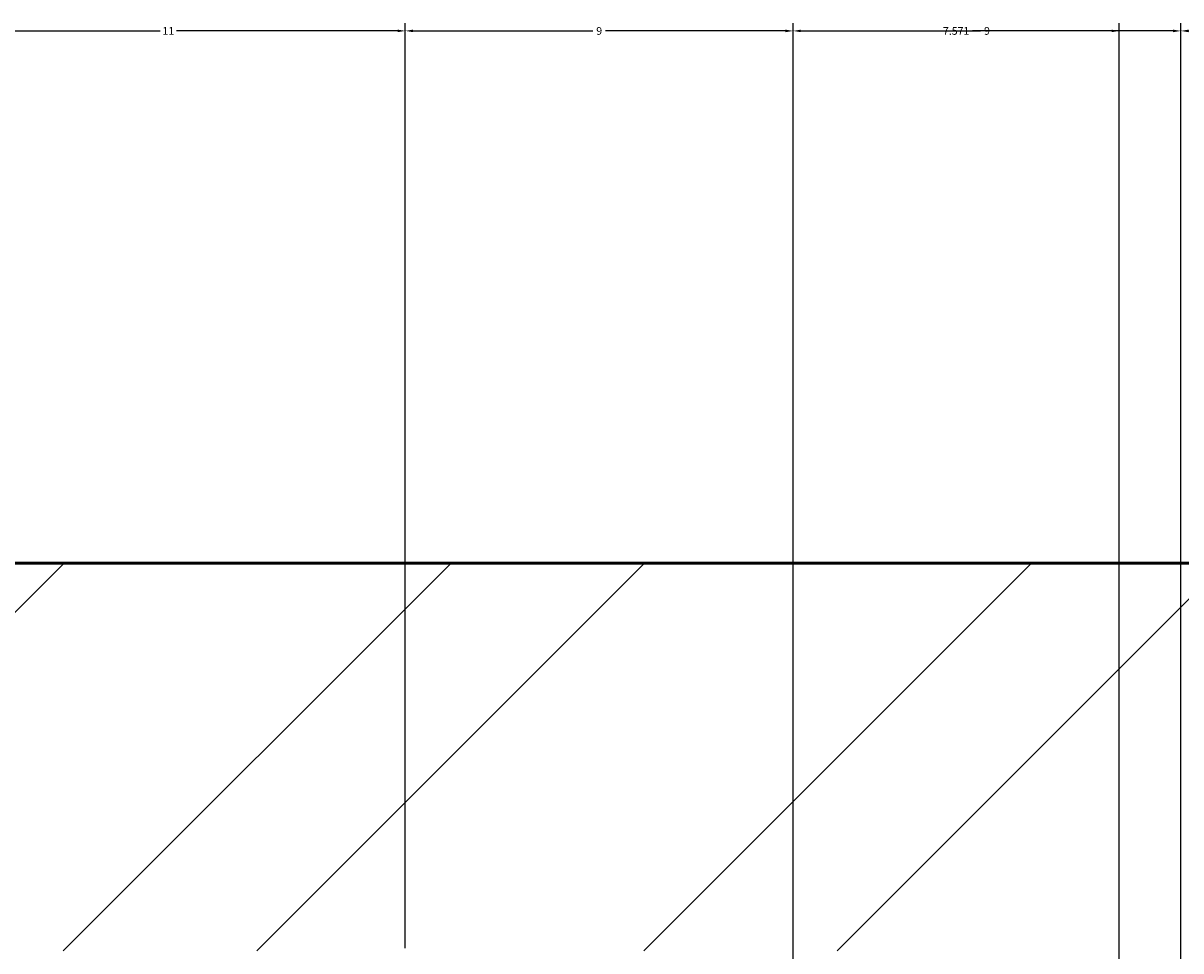
# Model space of a CAD drawing. Units: inches. Extents: x 2812 to 3051, y 1398 to 1659.
# Tile 63 of 65: x 2944 to 2970, y 1638 to 1659. Entities that reach past the tile are written whole.
import ezdxf

# ---------------------------------------------------------------- set-up
doc = ezdxf.new("R2010")
doc.units = ezdxf.units.IN
for name, color, linetype, lineweight in [('A-ANNO-DIMS', 2, 'Continuous', 18), ('S-CONC', 7, 'Continuous', 50), ('S-CONC-PATT', 8, 'Continuous', 18)]:
    doc.layers.add(name, color=color, linetype=linetype, lineweight=lineweight)
doc.styles.get("Standard").update_dxf_attribs({"font": 'arial.ttf'})
doc.dimstyles.get("Standard").update_dxf_attribs({"dimtxt": 0.18, "dimasz": 0.18, "dimexe": 0.18, "dimexo": 0.0625, "dimgap": 0.09, "dimtad": 0, "dimtih": 1, "dimtoh": 1, "dimdec": 4, "dimzin": 0, "dimdsep": 46, "dimtxsty": 'Standard', "dimcen": 0.09, "dimadec": 0, "dimazin": 0, "dimtfac": 1, "dimtdec": 4, "dimtofl": 0, "dimtmove": 0, "dimatfit": 3, "dimfxl": 1, "dimtolj": 1, "dimtzin": 0, "dimarcsym": 0})

# ---------------------------------------------------------------- blocks, each defined once
blk = doc.blocks.new('*D20')
at = {"layer": 'A-ANNO-DIMS', "color": 0, "lineweight": -2, "transparency": 16777216}
for p, q in [((2941.385, 1625.882), (2941.385, 1659.35)), ((2952.385, 1637.882), (2952.385, 1659.35)), ((2941.565, 1659.17), (2946.692, 1659.17)), ((2952.205, 1659.17), (2947.078, 1659.17))]:
    blk.add_line(p, q, dxfattribs=at)
at = {"layer": 'A-ANNO-DIMS', "color": 0, "transparency": 16777216}
for points in [[(2941.565, 1659.2), (2941.565, 1659.14), (2941.385, 1659.17)], [(2952.205, 1659.2), (2952.205, 1659.14), (2952.385, 1659.17)]]:
    blk.add_solid(points, dxfattribs=at)
at = {"layer": 'Defpoints', "color": 0, "transparency": 16777216}
for p in [(2952.385, 1659.17), (2952.385, 1637.82), (2941.385, 1625.82)]:
    blk.add_point(p, dxfattribs=at)
at = {"layer": 'A-ANNO-DIMS', "color": 0, "transparency": 16777216, "insert": (2946.885, 1659.17), "char_height": 0.18, "attachment_point": 5}
blk.add_mtext('\\A1;11', dxfattribs=at)
blk = doc.blocks.new('*D21')
at = {"layer": 'A-ANNO-DIMS', "color": 0, "lineweight": -2, "transparency": 16777216}
for p, q in [((2952.385, 1637.882), (2952.385, 1659.35)), ((2961.385, 1637.882), (2961.385, 1659.35)), ((2952.565, 1659.17), (2956.736, 1659.17)), ((2961.205, 1659.17), (2957.034, 1659.17))]:
    blk.add_line(p, q, dxfattribs=at)
at = {"layer": 'A-ANNO-DIMS', "color": 0, "transparency": 16777216}
for points in [[(2952.565, 1659.2), (2952.565, 1659.14), (2952.385, 1659.17)], [(2961.205, 1659.2), (2961.205, 1659.14), (2961.385, 1659.17)]]:
    blk.add_solid(points, dxfattribs=at)
at = {"layer": 'Defpoints', "color": 0, "transparency": 16777216}
for p in [(2961.385, 1659.17), (2952.385, 1637.82), (2961.385, 1637.82)]:
    blk.add_point(p, dxfattribs=at)
at = {"layer": 'A-ANNO-DIMS', "color": 0, "transparency": 16777216, "insert": (2956.885, 1659.17), "char_height": 0.18, "attachment_point": 5}
blk.add_mtext('\\A1;9', dxfattribs=at)
blk = doc.blocks.new('*D22')
at = {"layer": 'A-ANNO-DIMS', "color": 0, "lineweight": -2, "transparency": 16777216}
for p, q in [((2961.385, 1637.882), (2961.385, 1659.35)), ((2970.385, 1625.882), (2970.385, 1659.35)), ((2961.565, 1659.17), (2965.736, 1659.17)), ((2970.205, 1659.17), (2966.034, 1659.17))]:
    blk.add_line(p, q, dxfattribs=at)
at = {"layer": 'A-ANNO-DIMS', "color": 0, "transparency": 16777216}
for points in [[(2961.565, 1659.2), (2961.565, 1659.14), (2961.385, 1659.17)], [(2970.205, 1659.2), (2970.205, 1659.14), (2970.385, 1659.17)]]:
    blk.add_solid(points, dxfattribs=at)
at = {"layer": 'Defpoints', "color": 0, "transparency": 16777216}
for p in [(2970.385, 1659.17), (2961.385, 1637.82), (2970.385, 1625.82)]:
    blk.add_point(p, dxfattribs=at)
at = {"layer": 'A-ANNO-DIMS', "color": 0, "transparency": 16777216, "insert": (2965.885, 1659.17), "char_height": 0.18, "attachment_point": 5}
blk.add_mtext('\\A1;9', dxfattribs=at)
blk = doc.blocks.new('*D23')
at = {"layer": 'A-ANNO-DIMS', "color": 0, "lineweight": -2, "transparency": 16777216}
for p, q in [((2970.385, 1625.882), (2970.385, 1659.35)), ((2979.385, 1625.882), (2979.385, 1659.35)), ((2970.565, 1659.17), (2974.736, 1659.17)), ((2979.205, 1659.17), (2975.034, 1659.17))]:
    blk.add_line(p, q, dxfattribs=at)
at = {"layer": 'A-ANNO-DIMS', "color": 0, "transparency": 16777216}
for points in [[(2970.565, 1659.2), (2970.565, 1659.14), (2970.385, 1659.17)], [(2979.205, 1659.2), (2979.205, 1659.14), (2979.385, 1659.17)]]:
    blk.add_solid(points, dxfattribs=at)
at = {"layer": 'Defpoints', "color": 0, "transparency": 16777216}
for p in [(2979.385, 1659.17), (2970.385, 1625.82), (2979.385, 1625.82)]:
    blk.add_point(p, dxfattribs=at)
at = {"layer": 'A-ANNO-DIMS', "color": 0, "transparency": 16777216, "insert": (2974.885, 1659.17), "char_height": 0.18, "attachment_point": 5}
blk.add_mtext('\\A1;9', dxfattribs=at)
blk = doc.blocks.new('*D69')
at = {"layer": 'A-ANNO-DIMS', "color": 0, "lineweight": -2, "transparency": 16777216}
for p, q in [((2961.385, 1472.098), (2961.385, 1659.35)), ((2968.956, 1467.81), (2968.956, 1659.35)), ((2961.565, 1659.17), (2964.795, 1659.17)), ((2968.776, 1659.17), (2965.546, 1659.17))]:
    blk.add_line(p, q, dxfattribs=at)
at = {"layer": 'A-ANNO-DIMS', "color": 0, "transparency": 16777216}
for points in [[(2961.565, 1659.2), (2961.565, 1659.14), (2961.385, 1659.17)], [(2968.776, 1659.2), (2968.776, 1659.14), (2968.956, 1659.17)]]:
    blk.add_solid(points, dxfattribs=at)
at = {"layer": 'Defpoints', "color": 0, "transparency": 16777216}
for p in [(2968.956, 1659.17), (2961.385, 1472.035), (2968.956, 1467.747)]:
    blk.add_point(p, dxfattribs=at)
at = {"layer": 'A-ANNO-DIMS', "color": 0, "transparency": 16777216, "insert": (2965.17, 1659.17), "char_height": 0.18, "attachment_point": 5}
blk.add_mtext('\\A1;7.571', dxfattribs=at)

msp = doc.modelspace()

# ---------------------------------------------------------------- hatches: boundary and pattern name
at = {"layer": 'S-CONC-PATT'}
h = msp.add_hatch(dxfattribs=at)
h.set_pattern_fill('ANSI32', color=256)
h.paths.add_polyline_path([(3027.3849, 1646.82), (2835.3849, 1646.82), (2835.3849, 1603.2296), (2844.3849, 1603.2296), (2844.3849, 1637.82), (3018.3849, 1637.82), (3018.3849, 1602.5441), (3027.3849, 1602.5441)])
h.paths.add_polyline_path([(2844.3849, 1594.2296), (2835.3849, 1594.2296), (2835.3849, 1550.82), (3027.3849, 1550.82), (3027.3849, 1593.5441), (3018.3849, 1593.5441), (3018.3849, 1559.82), (2844.3849, 1559.82)])
h.paths.add_polyline_path([(2844.3849, 1482.0354), (2835.3849, 1482.0354), (2835.3849, 1463.4959), (2844.3849, 1463.4959)])
h.paths.add_polyline_path([(2844.3849, 1461.4959), (2835.3849, 1461.4959), (2835.3849, 1416.0354), (2844.3849, 1416.0354)])
h.paths.add_polyline_path([(3027.3849, 1482.0354), (3018.3849, 1482.0354), (3018.3849, 1463.2854), (3027.3849, 1463.2854)])
h.paths.add_polyline_path([(3027.3849, 1461.2854), (3018.3849, 1461.2854), (3018.3849, 1416.0354), (3027.3849, 1416.0354)])
h.paths.add_polyline_path([(2961.3849, 1448.4738), (2952.3849, 1448.4738), (2952.3849, 1416.0354), (2961.3849, 1416.0354)])
h.paths.add_polyline_path([(2961.3849, 1462.3026), (2952.3849, 1462.3026), (2952.3849, 1450.4738), (2961.3849, 1450.4738)])
h.paths.add_polyline_path([(2961.3849, 1472.0354), (2952.3849, 1472.0354), (2952.3849, 1462.3026), (2961.3849, 1462.3026)])

# ---------------------------------------------------------------- linework, layer by layer
at = {"layer": 'S-CONC'}
msp.add_line((2835.3849, 1646.82), (3027.3849, 1646.82), dxfattribs=at)

# ---------------------------------------------------------------- dimensions: what is measured, and where the dimension line sits
at = {"layer": 'A-ANNO-DIMS'}
for base, p1, p2, override, picture, middle in [((2952.3849, 1659.17), (2941.3849, 1625.82), (2952.3849, 1637.82), {"dimdec": 0, "dimlfac": 1, "dimrnd": 0, "dimzin": 0, "dimdsep": 46, "dimlunit": 2}, '*D20', (2946.8849, 1659.17)), ((2961.3849, 1659.17), (2952.3849, 1637.82), (2961.3849, 1637.82), {"dimdec": 0, "dimlfac": 1, "dimrnd": 0, "dimzin": 0, "dimdsep": 46, "dimlunit": 2}, '*D21', (2956.8849, 1659.17)), ((2970.3849, 1659.17), (2961.3849, 1637.82), (2970.3849, 1625.82), {"dimdec": 0, "dimlfac": 1, "dimrnd": 0, "dimzin": 0, "dimdsep": 46, "dimlunit": 2}, '*D22', (2965.8849, 1659.17)), ((2968.9558, 1659.17), (2961.3849, 1472.0354), (2968.9558, 1467.7474), {"dimdec": 3, "dimlfac": 1, "dimrnd": 0, "dimzin": 0, "dimdsep": 46, "dimlunit": 2}, '*D69', (2965.1704, 1659.17)), ((2979.3849, 1659.17), (2970.3849, 1625.82), (2979.3849, 1625.82), {"dimdec": 0, "dimlfac": 1, "dimrnd": 0, "dimzin": 0, "dimdsep": 46, "dimlunit": 2}, '*D23', (2974.8849, 1659.17))]:
    dim = msp.add_linear_dim(base=base, p1=p1, p2=p2, dimstyle='Standard', override=override, dxfattribs=at)
    dim.commit()
    dim.dimension.update_dxf_attribs({"geometry": picture, "text_midpoint": middle})

doc.saveas('drawing.dxf')
